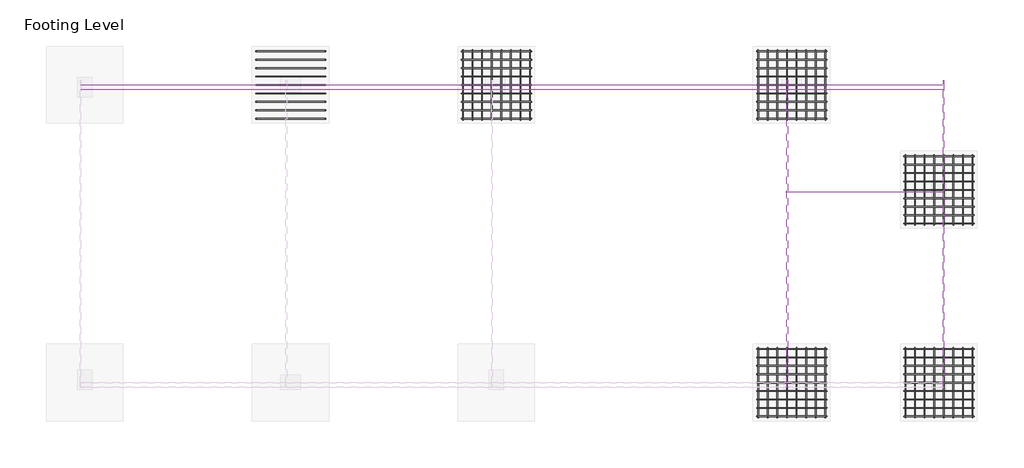
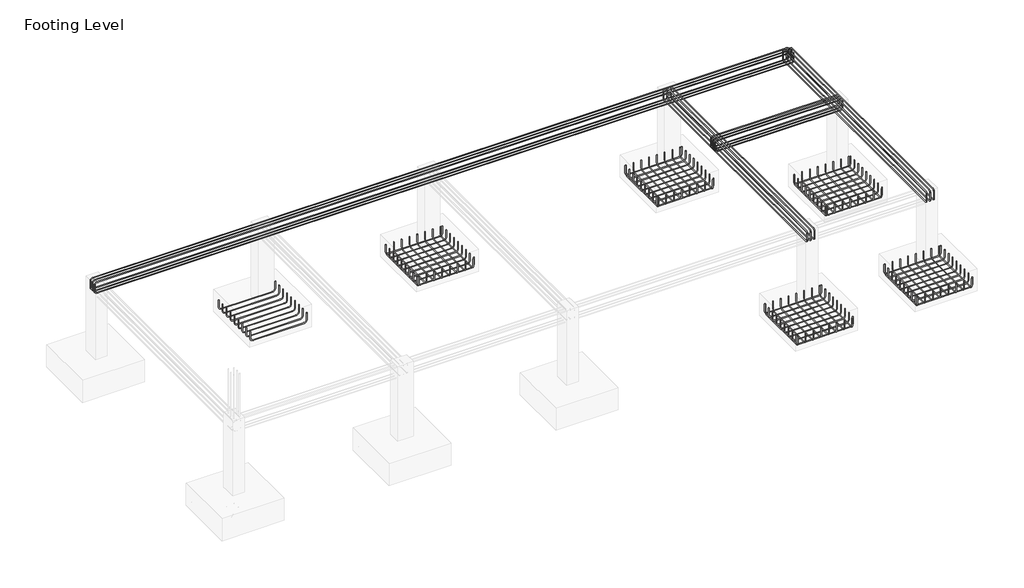
# One storey, part 3 of 3: 19 reinforcing bars.
"""IFC4 building model written with IfcOpenShell, lengths in millimetres."""

from ifc_helpers import new_model, si_unit, point, frame, origin, place, context, project, spatial, polyline, circle_curve, trimmed, segment, composite_curve, source, transform, mapped, element, save
from ifc_brep_helpers import swept_disk

model = new_model("IFC4")

# Units and contexts
model_context = context("Model", 3, world=origin())
ifc_project = project(units=[si_unit("LENGTHUNIT", "METRE", prefix="MILLI")], contexts=[model_context])

# Site, building, storey
site = spatial("IfcSite", under=ifc_project)
building = spatial("IfcBuilding", under=site)
storey = spatial("IfcBuildingStorey", under=building, Name="Footing Level", Elevation=-1524.0)

# Reinforcing bars
placement = place(None, origin())
reinforcing_bar_shape = source(origin(), model_context, "Body", "SolidModel", [
    swept_disk(composite_curve([segment(polyline([(2294.7534193, -243.2665369, -1724.0), (2294.7534193, -243.2665369, -1872.0)]), True, "CONTINUOUS"), segment(trimmed(circle_curve(frame((2294.7534193, -197.2665369, -1872.0), z_axis=(1.0, 0.0, 0.0), x_axis=(0.0, -46.0, 0.0)), 46.0), [point((2294.7534193, -243.2665369, -1872.0))], [point((2294.7534193, -197.2665369, -1918.0))], True, "CARTESIAN"), True, "CONTINUOUS"), segment(polyline([(2294.7534193, -197.2665369, -1918.0), (2294.7534193, 798.7334631, -1918.0)]), True, "CONTINUOUS"), segment(trimmed(circle_curve(frame((2294.7534193, 798.7334631, -1872.0), z_axis=(1.0, 0.0, 0.0), x_axis=(0.0, 0.0, -46.0)), 46.0), [point((2294.7534193, 798.7334631, -1918.0))], [point((2294.7534193, 844.7334631, -1872.0))], True, "CARTESIAN"), True, "CONTINUOUS"), segment(polyline([(2294.7534193, 844.7334631, -1872.0), (2294.7534193, 844.7334631, -1724.0)]), True, "CONTINUOUS")], self_intersect=False), 6.0),
])
element("IfcReinforcingBar", 1, at=placement, inside=storey, context=model_context, shape_type="MappedRepresentation", body=[
    mapped(reinforcing_bar_shape, transform((0.0, 0.0, 0.0), x_axis=(1.0, 0.0, 0.0), y_axis=(0.0, 1.0, 0.0), z_axis=(0.0, 0.0, 1.0))),
    mapped(reinforcing_bar_shape, transform((-149.7374868, 0.0, 0.0), x_axis=(1.0, 0.0, 0.0), y_axis=(0.0, 1.0, 0.0), z_axis=(0.0, 0.0, 1.0))),
    mapped(reinforcing_bar_shape, transform((-299.4749737, 0.0, 0.0), x_axis=(1.0, 0.0, 0.0), y_axis=(0.0, 1.0, 0.0), z_axis=(0.0, 0.0, 1.0))),
    mapped(reinforcing_bar_shape, transform((-449.2124605, 0.0, 0.0), x_axis=(1.0, 0.0, 0.0), y_axis=(0.0, 1.0, 0.0), z_axis=(0.0, 0.0, 1.0))),
    mapped(reinforcing_bar_shape, transform((-598.9499474, 0.0, 0.0), x_axis=(1.0, 0.0, 0.0), y_axis=(0.0, 1.0, 0.0), z_axis=(0.0, 0.0, 1.0))),
    mapped(reinforcing_bar_shape, transform((-748.6874342, 0.0, 0.0), x_axis=(1.0, 0.0, 0.0), y_axis=(0.0, 1.0, 0.0), z_axis=(0.0, 0.0, 1.0))),
    mapped(reinforcing_bar_shape, transform((-898.424921, 0.0, 0.0), x_axis=(1.0, 0.0, 0.0), y_axis=(0.0, 1.0, 0.0), z_axis=(0.0, 0.0, 1.0))),
    mapped(reinforcing_bar_shape, transform((-1048.1624079, 0.0, 0.0), x_axis=(1.0, 0.0, 0.0), y_axis=(0.0, 1.0, 0.0), z_axis=(0.0, 0.0, 1.0))),
])
reinforcing_bar_2_shape = source(origin(), model_context, "Body", "SolidModel", [
    swept_disk(composite_curve([segment(polyline([(1227.6882476, -224.7796689, -1711.15), (1227.6882476, -224.7796689, -1859.15)]), True, "CONTINUOUS"), segment(trimmed(circle_curve(frame((1273.6882476, -224.7796689, -1859.15), z_axis=(0.0, -1.0, 0.0), x_axis=(-46.0, 0.0, 0.0)), 46.0), [point((1227.6882476, -224.7796689, -1859.15))], [point((1273.6882476, -224.7796689, -1905.15))], True, "CARTESIAN"), True, "CONTINUOUS"), segment(polyline([(1273.6882476, -224.7796689, -1905.15), (2269.6882476, -224.7796689, -1905.15)]), True, "CONTINUOUS"), segment(trimmed(circle_curve(frame((2269.6882476, -224.7796689, -1859.15), z_axis=(0.0, -1.0, 0.0), x_axis=(0.0, 0.0, -46.0)), 46.0), [point((2269.6882476, -224.7796689, -1905.15))], [point((2315.6882476, -224.7796689, -1859.15))], True, "CARTESIAN"), True, "CONTINUOUS"), segment(polyline([(2315.6882476, -224.7796689, -1859.15), (2315.6882476, -224.7796689, -1711.15)]), True, "CONTINUOUS")], self_intersect=False), 6.0),
])
element("IfcReinforcingBar", 2, at=placement, inside=storey, context=model_context, shape_type="MappedRepresentation", body=[
    mapped(reinforcing_bar_2_shape, transform((0.0, 0.0, 0.0), x_axis=(1.0, 0.0, 0.0), y_axis=(0.0, 1.0, 0.0), z_axis=(0.0, 0.0, 1.0))),
    mapped(reinforcing_bar_2_shape, transform((0.0, 131.3537501, 0.0), x_axis=(1.0, 0.0, 0.0), y_axis=(0.0, 1.0, 0.0), z_axis=(0.0, 0.0, 1.0))),
    mapped(reinforcing_bar_2_shape, transform((0.0, 262.7075003, 0.0), x_axis=(1.0, 0.0, 0.0), y_axis=(0.0, 1.0, 0.0), z_axis=(0.0, 0.0, 1.0))),
    mapped(reinforcing_bar_2_shape, transform((0.0, 394.0612504, 0.0), x_axis=(1.0, 0.0, 0.0), y_axis=(0.0, 1.0, 0.0), z_axis=(0.0, 0.0, 1.0))),
    mapped(reinforcing_bar_2_shape, transform((0.0, 525.4150006, 0.0), x_axis=(1.0, 0.0, 0.0), y_axis=(0.0, 1.0, 0.0), z_axis=(0.0, 0.0, 1.0))),
    mapped(reinforcing_bar_2_shape, transform((0.0, 656.7687507, 0.0), x_axis=(1.0, 0.0, 0.0), y_axis=(0.0, 1.0, 0.0), z_axis=(0.0, 0.0, 1.0))),
    mapped(reinforcing_bar_2_shape, transform((0.0, 788.1225008, 0.0), x_axis=(1.0, 0.0, 0.0), y_axis=(0.0, 1.0, 0.0), z_axis=(0.0, 0.0, 1.0))),
    mapped(reinforcing_bar_2_shape, transform((0.0, 919.476251, 0.0), x_axis=(1.0, 0.0, 0.0), y_axis=(0.0, 1.0, 0.0), z_axis=(0.0, 0.0, 1.0))),
    mapped(reinforcing_bar_2_shape, transform((0.0, 1050.8300011, 0.0), x_axis=(1.0, 0.0, 0.0), y_axis=(0.0, 1.0, 0.0), z_axis=(0.0, 0.0, 1.0))),
])
reinforcing_bar_3_shape = source(origin(), model_context, "Body", "SolidModel", [
    swept_disk(composite_curve([segment(polyline([(4593.4534193, -243.2665369, -1724.0), (4593.4534193, -243.2665369, -1872.0)]), True, "CONTINUOUS"), segment(trimmed(circle_curve(frame((4593.4534193, -197.2665369, -1872.0), z_axis=(1.0, 0.0, 0.0), x_axis=(0.0, -46.0, 0.0)), 46.0), [point((4593.4534193, -243.2665369, -1872.0))], [point((4593.4534193, -197.2665369, -1918.0))], True, "CARTESIAN"), True, "CONTINUOUS"), segment(polyline([(4593.4534193, -197.2665369, -1918.0), (4593.4534193, 798.7334631, -1918.0)]), True, "CONTINUOUS"), segment(trimmed(circle_curve(frame((4593.4534193, 798.7334631, -1872.0), z_axis=(1.0, 0.0, 0.0), x_axis=(0.0, 0.0, -46.0)), 46.0), [point((4593.4534193, 798.7334631, -1918.0))], [point((4593.4534193, 844.7334631, -1872.0))], True, "CARTESIAN"), True, "CONTINUOUS"), segment(polyline([(4593.4534193, 844.7334631, -1872.0), (4593.4534193, 844.7334631, -1724.0)]), True, "CONTINUOUS")], self_intersect=False), 6.0),
])
element("IfcReinforcingBar", 3, at=placement, inside=storey, context=model_context, shape_type="MappedRepresentation", body=[
    mapped(reinforcing_bar_3_shape, transform((0.0, 0.0, 0.0), x_axis=(1.0, 0.0, 0.0), y_axis=(0.0, 1.0, 0.0), z_axis=(0.0, 0.0, 1.0))),
    mapped(reinforcing_bar_3_shape, transform((-149.7374868, 0.0, 0.0), x_axis=(1.0, 0.0, 0.0), y_axis=(0.0, 1.0, 0.0), z_axis=(0.0, 0.0, 1.0))),
    mapped(reinforcing_bar_3_shape, transform((-299.4749737, 0.0, 0.0), x_axis=(1.0, 0.0, 0.0), y_axis=(0.0, 1.0, 0.0), z_axis=(0.0, 0.0, 1.0))),
    mapped(reinforcing_bar_3_shape, transform((-449.2124605, 0.0, 0.0), x_axis=(1.0, 0.0, 0.0), y_axis=(0.0, 1.0, 0.0), z_axis=(0.0, 0.0, 1.0))),
    mapped(reinforcing_bar_3_shape, transform((-598.9499474, 0.0, 0.0), x_axis=(1.0, 0.0, 0.0), y_axis=(0.0, 1.0, 0.0), z_axis=(0.0, 0.0, 1.0))),
    mapped(reinforcing_bar_3_shape, transform((-748.6874342, 0.0, 0.0), x_axis=(1.0, 0.0, 0.0), y_axis=(0.0, 1.0, 0.0), z_axis=(0.0, 0.0, 1.0))),
    mapped(reinforcing_bar_3_shape, transform((-898.424921, 0.0, 0.0), x_axis=(1.0, 0.0, 0.0), y_axis=(0.0, 1.0, 0.0), z_axis=(0.0, 0.0, 1.0))),
    mapped(reinforcing_bar_3_shape, transform((-1048.1624079, 0.0, 0.0), x_axis=(1.0, 0.0, 0.0), y_axis=(0.0, 1.0, 0.0), z_axis=(0.0, 0.0, 1.0))),
])
reinforcing_bar_4_shape = source(origin(), model_context, "Body", "SolidModel", [
    swept_disk(composite_curve([segment(polyline([(3526.3882476, -224.7796689, -1711.15), (3526.3882476, -224.7796689, -1859.15)]), True, "CONTINUOUS"), segment(trimmed(circle_curve(frame((3572.3882476, -224.7796689, -1859.15), z_axis=(0.0, -1.0, 0.0), x_axis=(-46.0, 0.0, 0.0)), 46.0), [point((3526.3882476, -224.7796689, -1859.15))], [point((3572.3882476, -224.7796689, -1905.15))], True, "CARTESIAN"), True, "CONTINUOUS"), segment(polyline([(3572.3882476, -224.7796689, -1905.15), (4568.3882476, -224.7796689, -1905.15)]), True, "CONTINUOUS"), segment(trimmed(circle_curve(frame((4568.3882476, -224.7796689, -1859.15), z_axis=(0.0, -1.0, 0.0), x_axis=(0.0, 0.0, -46.0)), 46.0), [point((4568.3882476, -224.7796689, -1905.15))], [point((4614.3882476, -224.7796689, -1859.15))], True, "CARTESIAN"), True, "CONTINUOUS"), segment(polyline([(4614.3882476, -224.7796689, -1859.15), (4614.3882476, -224.7796689, -1711.15)]), True, "CONTINUOUS")], self_intersect=False), 6.0),
])
element("IfcReinforcingBar", 4, at=placement, inside=storey, context=model_context, shape_type="MappedRepresentation", body=[
    mapped(reinforcing_bar_4_shape, transform((0.0, 0.0, 0.0), x_axis=(1.0, 0.0, 0.0), y_axis=(0.0, 1.0, 0.0), z_axis=(0.0, 0.0, 1.0))),
    mapped(reinforcing_bar_4_shape, transform((0.0, 131.3537501, 0.0), x_axis=(1.0, 0.0, 0.0), y_axis=(0.0, 1.0, 0.0), z_axis=(0.0, 0.0, 1.0))),
    mapped(reinforcing_bar_4_shape, transform((0.0, 262.7075003, 0.0), x_axis=(1.0, 0.0, 0.0), y_axis=(0.0, 1.0, 0.0), z_axis=(0.0, 0.0, 1.0))),
    mapped(reinforcing_bar_4_shape, transform((0.0, 394.0612504, 0.0), x_axis=(1.0, 0.0, 0.0), y_axis=(0.0, 1.0, 0.0), z_axis=(0.0, 0.0, 1.0))),
    mapped(reinforcing_bar_4_shape, transform((0.0, 525.4150006, 0.0), x_axis=(1.0, 0.0, 0.0), y_axis=(0.0, 1.0, 0.0), z_axis=(0.0, 0.0, 1.0))),
    mapped(reinforcing_bar_4_shape, transform((0.0, 656.7687507, 0.0), x_axis=(1.0, 0.0, 0.0), y_axis=(0.0, 1.0, 0.0), z_axis=(0.0, 0.0, 1.0))),
    mapped(reinforcing_bar_4_shape, transform((0.0, 788.1225008, 0.0), x_axis=(1.0, 0.0, 0.0), y_axis=(0.0, 1.0, 0.0), z_axis=(0.0, 0.0, 1.0))),
    mapped(reinforcing_bar_4_shape, transform((0.0, 919.476251, 0.0), x_axis=(1.0, 0.0, 0.0), y_axis=(0.0, 1.0, 0.0), z_axis=(0.0, 0.0, 1.0))),
    mapped(reinforcing_bar_4_shape, transform((0.0, 1050.8300011, 0.0), x_axis=(1.0, 0.0, 0.0), y_axis=(0.0, 1.0, 0.0), z_axis=(0.0, 0.0, 1.0))),
])
reinforcing_bar_5_shape = source(origin(), model_context, "Body", "SolidModel", [
    swept_disk(composite_curve([segment(polyline([(4593.4534193, 2766.6334631, -1724.0), (4593.4534193, 2766.6334631, -1872.0)]), True, "CONTINUOUS"), segment(trimmed(circle_curve(frame((4593.4534193, 2812.6334631, -1872.0), z_axis=(1.0, 0.0, 0.0), x_axis=(0.0, -46.0, 0.0)), 46.0), [point((4593.4534193, 2766.6334631, -1872.0))], [point((4593.4534193, 2812.6334631, -1918.0))], True, "CARTESIAN"), True, "CONTINUOUS"), segment(polyline([(4593.4534193, 2812.6334631, -1918.0), (4593.4534193, 3808.6334631, -1918.0)]), True, "CONTINUOUS"), segment(trimmed(circle_curve(frame((4593.4534193, 3808.6334631, -1872.0), z_axis=(1.0, 0.0, 0.0), x_axis=(0.0, 0.0, -46.0)), 46.0), [point((4593.4534193, 3808.6334631, -1918.0))], [point((4593.4534193, 3854.6334631, -1872.0))], True, "CARTESIAN"), True, "CONTINUOUS"), segment(polyline([(4593.4534193, 3854.6334631, -1872.0), (4593.4534193, 3854.6334631, -1724.0)]), True, "CONTINUOUS")], self_intersect=False), 6.0),
])
element("IfcReinforcingBar", 5, at=placement, inside=storey, context=model_context, shape_type="MappedRepresentation", body=[
    mapped(reinforcing_bar_5_shape, transform((0.0, 0.0, 0.0), x_axis=(1.0, 0.0, 0.0), y_axis=(0.0, 1.0, 0.0), z_axis=(0.0, 0.0, 1.0))),
    mapped(reinforcing_bar_5_shape, transform((-149.7374868, 0.0, 0.0), x_axis=(1.0, 0.0, 0.0), y_axis=(0.0, 1.0, 0.0), z_axis=(0.0, 0.0, 1.0))),
    mapped(reinforcing_bar_5_shape, transform((-299.4749737, 0.0, 0.0), x_axis=(1.0, 0.0, 0.0), y_axis=(0.0, 1.0, 0.0), z_axis=(0.0, 0.0, 1.0))),
    mapped(reinforcing_bar_5_shape, transform((-449.2124605, 0.0, 0.0), x_axis=(1.0, 0.0, 0.0), y_axis=(0.0, 1.0, 0.0), z_axis=(0.0, 0.0, 1.0))),
    mapped(reinforcing_bar_5_shape, transform((-598.9499474, 0.0, 0.0), x_axis=(1.0, 0.0, 0.0), y_axis=(0.0, 1.0, 0.0), z_axis=(0.0, 0.0, 1.0))),
    mapped(reinforcing_bar_5_shape, transform((-748.6874342, 0.0, 0.0), x_axis=(1.0, 0.0, 0.0), y_axis=(0.0, 1.0, 0.0), z_axis=(0.0, 0.0, 1.0))),
    mapped(reinforcing_bar_5_shape, transform((-898.424921, 0.0, 0.0), x_axis=(1.0, 0.0, 0.0), y_axis=(0.0, 1.0, 0.0), z_axis=(0.0, 0.0, 1.0))),
    mapped(reinforcing_bar_5_shape, transform((-1048.1624079, 0.0, 0.0), x_axis=(1.0, 0.0, 0.0), y_axis=(0.0, 1.0, 0.0), z_axis=(0.0, 0.0, 1.0))),
])
reinforcing_bar_6_shape = source(origin(), model_context, "Body", "SolidModel", [
    swept_disk(composite_curve([segment(polyline([(3526.3882476, 2785.1203311, -1711.15), (3526.3882476, 2785.1203311, -1859.15)]), True, "CONTINUOUS"), segment(trimmed(circle_curve(frame((3572.3882476, 2785.1203311, -1859.15), z_axis=(0.0, -1.0, 0.0), x_axis=(-46.0, 0.0, 0.0)), 46.0), [point((3526.3882476, 2785.1203311, -1859.15))], [point((3572.3882476, 2785.1203311, -1905.15))], True, "CARTESIAN"), True, "CONTINUOUS"), segment(polyline([(3572.3882476, 2785.1203311, -1905.15), (4568.3882476, 2785.1203311, -1905.15)]), True, "CONTINUOUS"), segment(trimmed(circle_curve(frame((4568.3882476, 2785.1203311, -1859.15), z_axis=(0.0, -1.0, 0.0), x_axis=(0.0, 0.0, -46.0)), 46.0), [point((4568.3882476, 2785.1203311, -1905.15))], [point((4614.3882476, 2785.1203311, -1859.15))], True, "CARTESIAN"), True, "CONTINUOUS"), segment(polyline([(4614.3882476, 2785.1203311, -1859.15), (4614.3882476, 2785.1203311, -1711.15)]), True, "CONTINUOUS")], self_intersect=False), 6.0),
])
element("IfcReinforcingBar", 6, at=placement, inside=storey, context=model_context, shape_type="MappedRepresentation", body=[
    mapped(reinforcing_bar_6_shape, transform((0.0, 0.0, 0.0), x_axis=(1.0, 0.0, 0.0), y_axis=(0.0, 1.0, 0.0), z_axis=(0.0, 0.0, 1.0))),
    mapped(reinforcing_bar_6_shape, transform((0.0, 131.3537501, 0.0), x_axis=(1.0, 0.0, 0.0), y_axis=(0.0, 1.0, 0.0), z_axis=(0.0, 0.0, 1.0))),
    mapped(reinforcing_bar_6_shape, transform((0.0, 262.7075003, 0.0), x_axis=(1.0, 0.0, 0.0), y_axis=(0.0, 1.0, 0.0), z_axis=(0.0, 0.0, 1.0))),
    mapped(reinforcing_bar_6_shape, transform((0.0, 394.0612504, 0.0), x_axis=(1.0, 0.0, 0.0), y_axis=(0.0, 1.0, 0.0), z_axis=(0.0, 0.0, 1.0))),
    mapped(reinforcing_bar_6_shape, transform((0.0, 525.4150006, 0.0), x_axis=(1.0, 0.0, 0.0), y_axis=(0.0, 1.0, 0.0), z_axis=(0.0, 0.0, 1.0))),
    mapped(reinforcing_bar_6_shape, transform((0.0, 656.7687507, 0.0), x_axis=(1.0, 0.0, 0.0), y_axis=(0.0, 1.0, 0.0), z_axis=(0.0, 0.0, 1.0))),
    mapped(reinforcing_bar_6_shape, transform((0.0, 788.1225008, 0.0), x_axis=(1.0, 0.0, 0.0), y_axis=(0.0, 1.0, 0.0), z_axis=(0.0, 0.0, 1.0))),
    mapped(reinforcing_bar_6_shape, transform((0.0, 919.476251, 0.0), x_axis=(1.0, 0.0, 0.0), y_axis=(0.0, 1.0, 0.0), z_axis=(0.0, 0.0, 1.0))),
    mapped(reinforcing_bar_6_shape, transform((0.0, 1050.8300011, 0.0), x_axis=(1.0, 0.0, 0.0), y_axis=(0.0, 1.0, 0.0), z_axis=(0.0, 0.0, 1.0))),
])
reinforcing_bar_7_shape = source(origin(), model_context, "Body", "SolidModel", [
    swept_disk(composite_curve([segment(polyline([(2294.7534193, 4404.9334631, -1724.0), (2294.7534193, 4404.9334631, -1872.0)]), True, "CONTINUOUS"), segment(trimmed(circle_curve(frame((2294.7534193, 4450.9334631, -1872.0), z_axis=(1.0, 0.0, 0.0), x_axis=(0.0, -46.0, 0.0)), 46.0), [point((2294.7534193, 4404.9334631, -1872.0))], [point((2294.7534193, 4450.9334631, -1918.0))], True, "CARTESIAN"), True, "CONTINUOUS"), segment(polyline([(2294.7534193, 4450.9334631, -1918.0), (2294.7534193, 5446.9334631, -1918.0)]), True, "CONTINUOUS"), segment(trimmed(circle_curve(frame((2294.7534193, 5446.9334631, -1872.0), z_axis=(1.0, 0.0, 0.0), x_axis=(0.0, 0.0, -46.0)), 46.0), [point((2294.7534193, 5446.9334631, -1918.0))], [point((2294.7534193, 5492.9334631, -1872.0))], True, "CARTESIAN"), True, "CONTINUOUS"), segment(polyline([(2294.7534193, 5492.9334631, -1872.0), (2294.7534193, 5492.9334631, -1724.0)]), True, "CONTINUOUS")], self_intersect=False), 6.0),
])
element("IfcReinforcingBar", 7, at=placement, inside=storey, context=model_context, shape_type="MappedRepresentation", body=[
    mapped(reinforcing_bar_7_shape, transform((0.0, 0.0, 0.0), x_axis=(1.0, 0.0, 0.0), y_axis=(0.0, 1.0, 0.0), z_axis=(0.0, 0.0, 1.0))),
    mapped(reinforcing_bar_7_shape, transform((-149.7374868, 0.0, 0.0), x_axis=(1.0, 0.0, 0.0), y_axis=(0.0, 1.0, 0.0), z_axis=(0.0, 0.0, 1.0))),
    mapped(reinforcing_bar_7_shape, transform((-299.4749737, 0.0, 0.0), x_axis=(1.0, 0.0, 0.0), y_axis=(0.0, 1.0, 0.0), z_axis=(0.0, 0.0, 1.0))),
    mapped(reinforcing_bar_7_shape, transform((-449.2124605, 0.0, 0.0), x_axis=(1.0, 0.0, 0.0), y_axis=(0.0, 1.0, 0.0), z_axis=(0.0, 0.0, 1.0))),
    mapped(reinforcing_bar_7_shape, transform((-598.9499474, 0.0, 0.0), x_axis=(1.0, 0.0, 0.0), y_axis=(0.0, 1.0, 0.0), z_axis=(0.0, 0.0, 1.0))),
    mapped(reinforcing_bar_7_shape, transform((-748.6874342, 0.0, 0.0), x_axis=(1.0, 0.0, 0.0), y_axis=(0.0, 1.0, 0.0), z_axis=(0.0, 0.0, 1.0))),
    mapped(reinforcing_bar_7_shape, transform((-898.424921, 0.0, 0.0), x_axis=(1.0, 0.0, 0.0), y_axis=(0.0, 1.0, 0.0), z_axis=(0.0, 0.0, 1.0))),
    mapped(reinforcing_bar_7_shape, transform((-1048.1624079, 0.0, 0.0), x_axis=(1.0, 0.0, 0.0), y_axis=(0.0, 1.0, 0.0), z_axis=(0.0, 0.0, 1.0))),
])
reinforcing_bar_8_shape = source(origin(), model_context, "Body", "SolidModel", [
    swept_disk(composite_curve([segment(polyline([(1227.6882476, 4423.4203311, -1711.15), (1227.6882476, 4423.4203311, -1859.15)]), True, "CONTINUOUS"), segment(trimmed(circle_curve(frame((1273.6882476, 4423.4203311, -1859.15), z_axis=(0.0, -1.0, 0.0), x_axis=(-46.0, 0.0, 0.0)), 46.0), [point((1227.6882476, 4423.4203311, -1859.15))], [point((1273.6882476, 4423.4203311, -1905.15))], True, "CARTESIAN"), True, "CONTINUOUS"), segment(polyline([(1273.6882476, 4423.4203311, -1905.15), (2269.6882476, 4423.4203311, -1905.15)]), True, "CONTINUOUS"), segment(trimmed(circle_curve(frame((2269.6882476, 4423.4203311, -1859.15), z_axis=(0.0, -1.0, 0.0), x_axis=(0.0, 0.0, -46.0)), 46.0), [point((2269.6882476, 4423.4203311, -1905.15))], [point((2315.6882476, 4423.4203311, -1859.15))], True, "CARTESIAN"), True, "CONTINUOUS"), segment(polyline([(2315.6882476, 4423.4203311, -1859.15), (2315.6882476, 4423.4203311, -1711.15)]), True, "CONTINUOUS")], self_intersect=False), 6.0),
])
element("IfcReinforcingBar", 8, at=placement, inside=storey, context=model_context, shape_type="MappedRepresentation", body=[
    mapped(reinforcing_bar_8_shape, transform((0.0, 0.0, 0.0), x_axis=(1.0, 0.0, 0.0), y_axis=(0.0, 1.0, 0.0), z_axis=(0.0, 0.0, 1.0))),
    mapped(reinforcing_bar_8_shape, transform((0.0, 131.3537501, 0.0), x_axis=(1.0, 0.0, 0.0), y_axis=(0.0, 1.0, 0.0), z_axis=(0.0, 0.0, 1.0))),
    mapped(reinforcing_bar_8_shape, transform((0.0, 262.7075003, 0.0), x_axis=(1.0, 0.0, 0.0), y_axis=(0.0, 1.0, 0.0), z_axis=(0.0, 0.0, 1.0))),
    mapped(reinforcing_bar_8_shape, transform((0.0, 394.0612504, 0.0), x_axis=(1.0, 0.0, 0.0), y_axis=(0.0, 1.0, 0.0), z_axis=(0.0, 0.0, 1.0))),
    mapped(reinforcing_bar_8_shape, transform((0.0, 525.4150006, 0.0), x_axis=(1.0, 0.0, 0.0), y_axis=(0.0, 1.0, 0.0), z_axis=(0.0, 0.0, 1.0))),
    mapped(reinforcing_bar_8_shape, transform((0.0, 656.7687507, 0.0), x_axis=(1.0, 0.0, 0.0), y_axis=(0.0, 1.0, 0.0), z_axis=(0.0, 0.0, 1.0))),
    mapped(reinforcing_bar_8_shape, transform((0.0, 788.1225008, 0.0), x_axis=(1.0, 0.0, 0.0), y_axis=(0.0, 1.0, 0.0), z_axis=(0.0, 0.0, 1.0))),
    mapped(reinforcing_bar_8_shape, transform((0.0, 919.476251, 0.0), x_axis=(1.0, 0.0, 0.0), y_axis=(0.0, 1.0, 0.0), z_axis=(0.0, 0.0, 1.0))),
    mapped(reinforcing_bar_8_shape, transform((0.0, 1050.8300011, 0.0), x_axis=(1.0, 0.0, 0.0), y_axis=(0.0, 1.0, 0.0), z_axis=(0.0, 0.0, 1.0))),
])
reinforcing_bar_9_shape = source(origin(), model_context, "Body", "SolidModel", [
    swept_disk(composite_curve([segment(polyline([(-2315.3465807, 4404.9334631, -1724.0), (-2315.3465807, 4404.9334631, -1872.0)]), True, "CONTINUOUS"), segment(trimmed(circle_curve(frame((-2315.3465807, 4450.9334631, -1872.0), z_axis=(1.0, 0.0, 0.0), x_axis=(0.0, -46.0, 0.0)), 46.0), [point((-2315.3465807, 4404.9334631, -1872.0))], [point((-2315.3465807, 4450.9334631, -1918.0))], True, "CARTESIAN"), True, "CONTINUOUS"), segment(polyline([(-2315.3465807, 4450.9334631, -1918.0), (-2315.3465807, 5446.9334631, -1918.0)]), True, "CONTINUOUS"), segment(trimmed(circle_curve(frame((-2315.3465807, 5446.9334631, -1872.0), z_axis=(1.0, 0.0, 0.0), x_axis=(0.0, 0.0, -46.0)), 46.0), [point((-2315.3465807, 5446.9334631, -1918.0))], [point((-2315.3465807, 5492.9334631, -1872.0))], True, "CARTESIAN"), True, "CONTINUOUS"), segment(polyline([(-2315.3465807, 5492.9334631, -1872.0), (-2315.3465807, 5492.9334631, -1724.0)]), True, "CONTINUOUS")], self_intersect=False), 6.0),
])
element("IfcReinforcingBar", 9, at=placement, inside=storey, context=model_context, shape_type="MappedRepresentation", body=[
    mapped(reinforcing_bar_9_shape, transform((0.0, 0.0, 0.0), x_axis=(1.0, 0.0, 0.0), y_axis=(0.0, 1.0, 0.0), z_axis=(0.0, 0.0, 1.0))),
    mapped(reinforcing_bar_9_shape, transform((-149.7374868, 0.0, 0.0), x_axis=(1.0, 0.0, 0.0), y_axis=(0.0, 1.0, 0.0), z_axis=(0.0, 0.0, 1.0))),
    mapped(reinforcing_bar_9_shape, transform((-299.4749737, 0.0, 0.0), x_axis=(1.0, 0.0, 0.0), y_axis=(0.0, 1.0, 0.0), z_axis=(0.0, 0.0, 1.0))),
    mapped(reinforcing_bar_9_shape, transform((-449.2124605, 0.0, 0.0), x_axis=(1.0, 0.0, 0.0), y_axis=(0.0, 1.0, 0.0), z_axis=(0.0, 0.0, 1.0))),
    mapped(reinforcing_bar_9_shape, transform((-598.9499474, 0.0, 0.0), x_axis=(1.0, 0.0, 0.0), y_axis=(0.0, 1.0, 0.0), z_axis=(0.0, 0.0, 1.0))),
    mapped(reinforcing_bar_9_shape, transform((-748.6874342, 0.0, 0.0), x_axis=(1.0, 0.0, 0.0), y_axis=(0.0, 1.0, 0.0), z_axis=(0.0, 0.0, 1.0))),
    mapped(reinforcing_bar_9_shape, transform((-898.424921, 0.0, 0.0), x_axis=(1.0, 0.0, 0.0), y_axis=(0.0, 1.0, 0.0), z_axis=(0.0, 0.0, 1.0))),
    mapped(reinforcing_bar_9_shape, transform((-1048.1624079, 0.0, 0.0), x_axis=(1.0, 0.0, 0.0), y_axis=(0.0, 1.0, 0.0), z_axis=(0.0, 0.0, 1.0))),
])
reinforcing_bar_10_shape = source(origin(), model_context, "Body", "SolidModel", [
    swept_disk(composite_curve([segment(polyline([(-3382.4117524, 4423.4203311, -1711.15), (-3382.4117524, 4423.4203311, -1859.15)]), True, "CONTINUOUS"), segment(trimmed(circle_curve(frame((-3336.4117524, 4423.4203311, -1859.15), z_axis=(0.0, -1.0, 0.0), x_axis=(-46.0, 0.0, 0.0)), 46.0), [point((-3382.4117524, 4423.4203311, -1859.15))], [point((-3336.4117524, 4423.4203311, -1905.15))], True, "CARTESIAN"), True, "CONTINUOUS"), segment(polyline([(-3336.4117524, 4423.4203311, -1905.15), (-2340.4117524, 4423.4203311, -1905.15)]), True, "CONTINUOUS"), segment(trimmed(circle_curve(frame((-2340.4117524, 4423.4203311, -1859.15), z_axis=(0.0, -1.0, 0.0), x_axis=(0.0, 0.0, -46.0)), 46.0), [point((-2340.4117524, 4423.4203311, -1905.15))], [point((-2294.4117524, 4423.4203311, -1859.15))], True, "CARTESIAN"), True, "CONTINUOUS"), segment(polyline([(-2294.4117524, 4423.4203311, -1859.15), (-2294.4117524, 4423.4203311, -1711.15)]), True, "CONTINUOUS")], self_intersect=False), 6.0),
])
element("IfcReinforcingBar", 10, at=placement, inside=storey, context=model_context, shape_type="MappedRepresentation", body=[
    mapped(reinforcing_bar_10_shape, transform((0.0, 0.0, 0.0), x_axis=(1.0, 0.0, 0.0), y_axis=(0.0, 1.0, 0.0), z_axis=(0.0, 0.0, 1.0))),
    mapped(reinforcing_bar_10_shape, transform((0.0, 131.3537501, 0.0), x_axis=(1.0, 0.0, 0.0), y_axis=(0.0, 1.0, 0.0), z_axis=(0.0, 0.0, 1.0))),
    mapped(reinforcing_bar_10_shape, transform((0.0, 262.7075003, 0.0), x_axis=(1.0, 0.0, 0.0), y_axis=(0.0, 1.0, 0.0), z_axis=(0.0, 0.0, 1.0))),
    mapped(reinforcing_bar_10_shape, transform((0.0, 394.0612504, 0.0), x_axis=(1.0, 0.0, 0.0), y_axis=(0.0, 1.0, 0.0), z_axis=(0.0, 0.0, 1.0))),
    mapped(reinforcing_bar_10_shape, transform((0.0, 525.4150006, 0.0), x_axis=(1.0, 0.0, 0.0), y_axis=(0.0, 1.0, 0.0), z_axis=(0.0, 0.0, 1.0))),
    mapped(reinforcing_bar_10_shape, transform((0.0, 656.7687507, 0.0), x_axis=(1.0, 0.0, 0.0), y_axis=(0.0, 1.0, 0.0), z_axis=(0.0, 0.0, 1.0))),
    mapped(reinforcing_bar_10_shape, transform((0.0, 788.1225008, 0.0), x_axis=(1.0, 0.0, 0.0), y_axis=(0.0, 1.0, 0.0), z_axis=(0.0, 0.0, 1.0))),
    mapped(reinforcing_bar_10_shape, transform((0.0, 919.476251, 0.0), x_axis=(1.0, 0.0, 0.0), y_axis=(0.0, 1.0, 0.0), z_axis=(0.0, 0.0, 1.0))),
    mapped(reinforcing_bar_10_shape, transform((0.0, 1050.8300011, 0.0), x_axis=(1.0, 0.0, 0.0), y_axis=(0.0, 1.0, 0.0), z_axis=(0.0, 0.0, 1.0))),
])
reinforcing_bar_11_shape = source(origin(), model_context, "Body", "SolidModel", [
    swept_disk(composite_curve([segment(polyline([(-6595.5117524, 4423.4203311, -1711.15), (-6595.5117524, 4423.4203311, -1859.15)]), True, "CONTINUOUS"), segment(trimmed(circle_curve(frame((-6549.5117524, 4423.4203311, -1859.15), z_axis=(0.0, -1.0, 0.0), x_axis=(-46.0, 0.0, 0.0)), 46.0), [point((-6595.5117524, 4423.4203311, -1859.15))], [point((-6549.5117524, 4423.4203311, -1905.15))], True, "CARTESIAN"), True, "CONTINUOUS"), segment(polyline([(-6549.5117524, 4423.4203311, -1905.15), (-5553.5117524, 4423.4203311, -1905.15)]), True, "CONTINUOUS"), segment(trimmed(circle_curve(frame((-5553.5117524, 4423.4203311, -1859.15), z_axis=(0.0, -1.0, 0.0), x_axis=(0.0, 0.0, -46.0)), 46.0), [point((-5553.5117524, 4423.4203311, -1905.15))], [point((-5507.5117524, 4423.4203311, -1859.15))], True, "CARTESIAN"), True, "CONTINUOUS"), segment(polyline([(-5507.5117524, 4423.4203311, -1859.15), (-5507.5117524, 4423.4203311, -1711.15)]), True, "CONTINUOUS")], self_intersect=False), 6.0),
])
element("IfcReinforcingBar", 11, at=placement, inside=storey, context=model_context, shape_type="MappedRepresentation", body=[
    mapped(reinforcing_bar_11_shape, transform((0.0, 0.0, 0.0), x_axis=(1.0, 0.0, 0.0), y_axis=(0.0, 1.0, 0.0), z_axis=(0.0, 0.0, 1.0))),
    mapped(reinforcing_bar_11_shape, transform((0.0, 131.3537501, 0.0), x_axis=(1.0, 0.0, 0.0), y_axis=(0.0, 1.0, 0.0), z_axis=(0.0, 0.0, 1.0))),
    mapped(reinforcing_bar_11_shape, transform((0.0, 262.7075003, 0.0), x_axis=(1.0, 0.0, 0.0), y_axis=(0.0, 1.0, 0.0), z_axis=(0.0, 0.0, 1.0))),
    mapped(reinforcing_bar_11_shape, transform((0.0, 394.0612504, 0.0), x_axis=(1.0, 0.0, 0.0), y_axis=(0.0, 1.0, 0.0), z_axis=(0.0, 0.0, 1.0))),
    mapped(reinforcing_bar_11_shape, transform((0.0, 525.4150006, 0.0), x_axis=(1.0, 0.0, 0.0), y_axis=(0.0, 1.0, 0.0), z_axis=(0.0, 0.0, 1.0))),
    mapped(reinforcing_bar_11_shape, transform((0.0, 656.7687507, 0.0), x_axis=(1.0, 0.0, 0.0), y_axis=(0.0, 1.0, 0.0), z_axis=(0.0, 0.0, 1.0))),
    mapped(reinforcing_bar_11_shape, transform((0.0, 788.1225008, 0.0), x_axis=(1.0, 0.0, 0.0), y_axis=(0.0, 1.0, 0.0), z_axis=(0.0, 0.0, 1.0))),
    mapped(reinforcing_bar_11_shape, transform((0.0, 919.476251, 0.0), x_axis=(1.0, 0.0, 0.0), y_axis=(0.0, 1.0, 0.0), z_axis=(0.0, 0.0, 1.0))),
    mapped(reinforcing_bar_11_shape, transform((0.0, 1050.8300011, 0.0), x_axis=(1.0, 0.0, 0.0), y_axis=(0.0, 1.0, 0.0), z_axis=(0.0, 0.0, 1.0))),
])
reinforcing_bar_12_shape = source(origin(), model_context, "Body", "SolidModel", [
    swept_disk(composite_curve([segment(polyline([(1700.4887526, 5017.2334631, -237.1005051), (1700.4887526, 5017.2334631, -89.1005051)]), True, "CONTINUOUS"), segment(trimmed(circle_curve(frame((1700.4887526, 4971.2334631, -89.1005051), z_axis=(1.0, 0.0, 0.0), x_axis=(0.0, 46.0, 0.0)), 46.0), [point((1700.4887526, 5017.2334631, -89.1005051))], [point((1700.4887526, 4971.2334631, -43.1005051))], True, "CARTESIAN"), True, "CONTINUOUS"), segment(polyline([(1700.4887526, 4971.2334631, -43.1005051), (1700.4887526, 278.4334631, -43.1005051)]), True, "CONTINUOUS"), segment(trimmed(circle_curve(frame((1700.4887526, 278.4334631, -89.1005051), z_axis=(1.0, 0.0, 0.0), x_axis=(0.0, 0.0, 46.00000000000001)), 46.0), [point((1700.4887526, 278.4334631, -43.1005051))], [point((1700.4887526, 232.4334631, -89.1005051))], True, "CARTESIAN"), True, "CONTINUOUS"), segment(polyline([(1700.4887526, 232.4334631, -89.1005051), (1700.4887526, 232.4334631, -237.1005051)]), True, "CONTINUOUS")], self_intersect=False), 6.0),
])
element("IfcReinforcingBar", 12, at=placement, inside=storey, context=model_context, shape_type="MappedRepresentation", body=[
    mapped(reinforcing_bar_12_shape, transform((0.0, 0.0, 0.0), x_axis=(1.0, 0.0, 0.0), y_axis=(0.0, 1.0, 0.0), z_axis=(0.0, 0.0, 1.0))),
    mapped(reinforcing_bar_12_shape, transform((71.1994949, 0.0, 0.0), x_axis=(1.0, 0.0, 0.0), y_axis=(0.0, 1.0, 0.0), z_axis=(0.0, 0.0, 1.0))),
    mapped(reinforcing_bar_12_shape, transform((142.3989899, 0.0, 0.0), x_axis=(1.0, 0.0, 0.0), y_axis=(0.0, 1.0, 0.0), z_axis=(0.0, 0.0, 1.0))),
])
reinforcing_bar_13_shape = source(origin(), model_context, "Body", "SolidModel", [
    swept_disk(composite_curve([segment(polyline([(1700.4887526, 5017.2334631, -67.6994949), (1700.4887526, 5017.2334631, -215.6994949)]), True, "CONTINUOUS"), segment(trimmed(circle_curve(frame((1700.4887526, 4971.2334631, -215.6994949), z_axis=(-1.0, 0.0, 0.0), x_axis=(0.0, 46.0, 0.0)), 46.0), [point((1700.4887526, 5017.2334631, -215.6994949))], [point((1700.4887526, 4971.2334631, -261.6994949))], True, "CARTESIAN"), True, "CONTINUOUS"), segment(polyline([(1700.4887526, 4971.2334631, -261.6994949), (1700.4887526, 278.4334631, -261.6994949)]), True, "CONTINUOUS"), segment(trimmed(circle_curve(frame((1700.4887526, 278.4334631, -215.6994949), z_axis=(-1.0, 0.0, 0.0), x_axis=(0.0, 0.0, -46.0)), 46.0), [point((1700.4887526, 278.4334631, -261.6994949))], [point((1700.4887526, 232.4334631, -215.6994949))], True, "CARTESIAN"), True, "CONTINUOUS"), segment(polyline([(1700.4887526, 232.4334631, -215.6994949), (1700.4887526, 232.4334631, -67.6994949)]), True, "CONTINUOUS")], self_intersect=False), 6.0),
])
element("IfcReinforcingBar", 13, at=placement, inside=storey, context=model_context, shape_type="MappedRepresentation", body=[
    mapped(reinforcing_bar_13_shape, transform((0.0, 0.0, 0.0), x_axis=(1.0, 0.0, 0.0), y_axis=(0.0, 1.0, 0.0), z_axis=(0.0, 0.0, 1.0))),
    mapped(reinforcing_bar_13_shape, transform((71.1994949, 0.0, 0.0), x_axis=(1.0, 0.0, 0.0), y_axis=(0.0, 1.0, 0.0), z_axis=(0.0, 0.0, 1.0))),
    mapped(reinforcing_bar_13_shape, transform((142.3989899, 0.0, 0.0), x_axis=(1.0, 0.0, 0.0), y_axis=(0.0, 1.0, 0.0), z_axis=(0.0, 0.0, 1.0))),
])
reinforcing_bar_14_shape = source(origin(), model_context, "Body", "SolidModel", [
    swept_disk(composite_curve([segment(polyline([(3999.1887526, 5017.2334631, -237.1005051), (3999.1887526, 5017.2334631, -89.1005051)]), True, "CONTINUOUS"), segment(trimmed(circle_curve(frame((3999.1887526, 4971.2334631, -89.1005051), z_axis=(1.0, 0.0, 0.0), x_axis=(0.0, 46.0, 0.0)), 46.0), [point((3999.1887526, 5017.2334631, -89.1005051))], [point((3999.1887526, 4971.2334631, -43.1005051))], True, "CARTESIAN"), True, "CONTINUOUS"), segment(polyline([(3999.1887526, 4971.2334631, -43.1005051), (3999.1887526, 278.4334631, -43.1005051)]), True, "CONTINUOUS"), segment(trimmed(circle_curve(frame((3999.1887526, 278.4334631, -89.1005051), z_axis=(1.0, 0.0, 0.0), x_axis=(0.0, 0.0, 46.00000000000001)), 46.0), [point((3999.1887526, 278.4334631, -43.1005051))], [point((3999.1887526, 232.4334631, -89.1005051))], True, "CARTESIAN"), True, "CONTINUOUS"), segment(polyline([(3999.1887526, 232.4334631, -89.1005051), (3999.1887526, 232.4334631, -237.1005051)]), True, "CONTINUOUS")], self_intersect=False), 6.0),
])
element("IfcReinforcingBar", 14, at=placement, inside=storey, context=model_context, shape_type="MappedRepresentation", body=[
    mapped(reinforcing_bar_14_shape, transform((0.0, 0.0, 0.0), x_axis=(1.0, 0.0, 0.0), y_axis=(0.0, 1.0, 0.0), z_axis=(0.0, 0.0, 1.0))),
    mapped(reinforcing_bar_14_shape, transform((71.1994949, 0.0, 0.0), x_axis=(1.0, 0.0, 0.0), y_axis=(0.0, 1.0, 0.0), z_axis=(0.0, 0.0, 1.0))),
    mapped(reinforcing_bar_14_shape, transform((142.3989899, 0.0, 0.0), x_axis=(1.0, 0.0, 0.0), y_axis=(0.0, 1.0, 0.0), z_axis=(0.0, 0.0, 1.0))),
])
reinforcing_bar_15_shape = source(origin(), model_context, "Body", "SolidModel", [
    swept_disk(composite_curve([segment(polyline([(3999.1887526, 5017.2334631, -67.6994949), (3999.1887526, 5017.2334631, -215.6994949)]), True, "CONTINUOUS"), segment(trimmed(circle_curve(frame((3999.1887526, 4971.2334631, -215.6994949), z_axis=(-1.0, 0.0, 0.0), x_axis=(0.0, 46.0, 0.0)), 46.0), [point((3999.1887526, 5017.2334631, -215.6994949))], [point((3999.1887526, 4971.2334631, -261.6994949))], True, "CARTESIAN"), True, "CONTINUOUS"), segment(polyline([(3999.1887526, 4971.2334631, -261.6994949), (3999.1887526, 278.4334631, -261.6994949)]), True, "CONTINUOUS"), segment(trimmed(circle_curve(frame((3999.1887526, 278.4334631, -215.6994949), z_axis=(-1.0, 0.0, 0.0), x_axis=(0.0, 0.0, -46.0)), 46.0), [point((3999.1887526, 278.4334631, -261.6994949))], [point((3999.1887526, 232.4334631, -215.6994949))], True, "CARTESIAN"), True, "CONTINUOUS"), segment(polyline([(3999.1887526, 232.4334631, -215.6994949), (3999.1887526, 232.4334631, -67.6994949)]), True, "CONTINUOUS")], self_intersect=False), 6.0),
])
element("IfcReinforcingBar", 15, at=placement, inside=storey, context=model_context, shape_type="MappedRepresentation", body=[
    mapped(reinforcing_bar_15_shape, transform((0.0, 0.0, 0.0), x_axis=(1.0, 0.0, 0.0), y_axis=(0.0, 1.0, 0.0), z_axis=(0.0, 0.0, 1.0))),
    mapped(reinforcing_bar_15_shape, transform((71.1994949, 0.0, 0.0), x_axis=(1.0, 0.0, 0.0), y_axis=(0.0, 1.0, 0.0), z_axis=(0.0, 0.0, 1.0))),
    mapped(reinforcing_bar_15_shape, transform((142.3989899, 0.0, 0.0), x_axis=(1.0, 0.0, 0.0), y_axis=(0.0, 1.0, 0.0), z_axis=(0.0, 0.0, 1.0))),
])
reinforcing_bar_16_shape = source(origin(), model_context, "Body", "SolidModel", [
    swept_disk(composite_curve([segment(polyline([(-9325.7296265, 4877.7339681, -237.1005051), (-9325.7296265, 4877.7339681, -89.1005051)]), True, "CONTINUOUS"), segment(trimmed(circle_curve(frame((-9279.7296265, 4877.7339681, -89.1005051), z_axis=(0.0, 1.0, 0.0), x_axis=(-46.0, 0.0, 0.0)), 46.0), [point((-9325.7296265, 4877.7339681, -89.1005051))], [point((-9279.7296265, 4877.7339681, -43.1005051))], True, "CARTESIAN"), True, "CONTINUOUS"), segment(polyline([(-9279.7296265, 4877.7339681, -43.1005051), (4070.8650323, 4877.7339681, -43.1005051)]), True, "CONTINUOUS"), segment(trimmed(circle_curve(frame((4070.8650323, 4877.7339681, -89.1005051), z_axis=(0.0, 1.0, 0.0), x_axis=(0.0, 0.0, 46.00000000000001)), 46.0), [point((4070.8650323, 4877.7339681, -43.1005051))], [point((4116.8650323, 4877.7339681, -89.1005051))], True, "CARTESIAN"), True, "CONTINUOUS"), segment(polyline([(4116.8650323, 4877.7339681, -89.1005051), (4116.8650323, 4877.7339681, -237.1005051)]), True, "CONTINUOUS")], self_intersect=False), 6.0),
])
element("IfcReinforcingBar", 16, at=placement, inside=storey, context=model_context, shape_type="MappedRepresentation", body=[
    mapped(reinforcing_bar_16_shape, transform((0.0, 0.0, 0.0), x_axis=(1.0, 0.0, 0.0), y_axis=(0.0, 1.0, 0.0), z_axis=(0.0, 0.0, 1.0))),
    mapped(reinforcing_bar_16_shape, transform((0.0, 71.1994949, 0.0), x_axis=(1.0, 0.0, 0.0), y_axis=(0.0, 1.0, 0.0), z_axis=(0.0, 0.0, 1.0))),
    mapped(reinforcing_bar_16_shape, transform((0.0, 142.3989899, 0.0), x_axis=(1.0, 0.0, 0.0), y_axis=(0.0, 1.0, 0.0), z_axis=(0.0, 0.0, 1.0))),
])
reinforcing_bar_17_shape = source(origin(), model_context, "Body", "SolidModel", [
    swept_disk(composite_curve([segment(polyline([(-9326.1203644, 4877.7339681, -67.6994949), (-9326.1203644, 4877.7339681, -215.6994949)]), True, "CONTINUOUS"), segment(trimmed(circle_curve(frame((-9280.1203644, 4877.7339681, -215.6994949), z_axis=(0.0, -1.0, 0.0), x_axis=(-46.0, 0.0, 0.0)), 46.0), [point((-9326.1203644, 4877.7339681, -215.6994949))], [point((-9280.1203644, 4877.7339681, -261.6994949))], True, "CARTESIAN"), True, "CONTINUOUS"), segment(polyline([(-9280.1203644, 4877.7339681, -261.6994949), (4076.5679264, 4877.7339681, -261.6994949)]), True, "CONTINUOUS"), segment(trimmed(circle_curve(frame((4076.5679264, 4877.7339681, -215.6994949), z_axis=(0.0, -1.0, 0.0), x_axis=(0.0, 0.0, -46.0)), 46.0), [point((4076.5679264, 4877.7339681, -261.6994949))], [point((4122.5679264, 4877.7339681, -215.6994949))], True, "CARTESIAN"), True, "CONTINUOUS"), segment(polyline([(4122.5679264, 4877.7339681, -215.6994949), (4122.5679264, 4877.7339681, -67.6994949)]), True, "CONTINUOUS")], self_intersect=False), 6.0),
])
element("IfcReinforcingBar", 17, at=placement, inside=storey, context=model_context, shape_type="MappedRepresentation", body=[
    mapped(reinforcing_bar_17_shape, transform((0.0, 0.0, 0.0), x_axis=(1.0, 0.0, 0.0), y_axis=(0.0, 1.0, 0.0), z_axis=(0.0, 0.0, 1.0))),
    mapped(reinforcing_bar_17_shape, transform((0.0, 71.1994949, 0.0), x_axis=(1.0, 0.0, 0.0), y_axis=(0.0, 1.0, 0.0), z_axis=(0.0, 0.0, 1.0))),
    mapped(reinforcing_bar_17_shape, transform((0.0, 142.3989899, 0.0), x_axis=(1.0, 0.0, 0.0), y_axis=(0.0, 1.0, 0.0), z_axis=(0.0, 0.0, 1.0))),
])
reinforcing_bar_18_shape = source(origin(), model_context, "Body", "SolidModel", [
    swept_disk(composite_curve([segment(polyline([(4138.6882476, 3279.2814555, -238.8479924), (4138.6882476, 3279.2814555, -90.8479924)]), True, "CONTINUOUS"), segment(trimmed(circle_curve(frame((4092.6882476, 3279.2814555, -90.8479924), z_axis=(0.0, -1.0, 0.0), x_axis=(46.0, 0.0, 0.0)), 46.0), [point((4138.6882476, 3279.2814555, -90.8479924))], [point((4092.6882476, 3279.2814555, -44.8479924))], True, "CARTESIAN"), True, "CONTINUOUS"), segment(polyline([(4092.6882476, 3279.2814555, -44.8479924), (1734.3882476, 3279.2814555, -44.8479924)]), True, "CONTINUOUS"), segment(trimmed(circle_curve(frame((1734.3882476, 3279.2814555, -90.8479924), z_axis=(0.0, -1.0, 0.0), x_axis=(0.0, 0.0, 45.99999999999999)), 46.0), [point((1734.3882476, 3279.2814555, -44.8479924))], [point((1688.3882476, 3279.2814555, -90.8479924))], True, "CARTESIAN"), True, "CONTINUOUS"), segment(polyline([(1688.3882476, 3279.2814555, -90.8479924), (1688.3882476, 3279.2814555, -238.8479924)]), True, "CONTINUOUS")], self_intersect=False), 6.0),
])
element("IfcReinforcingBar", 18, at=placement, inside=storey, context=model_context, shape_type="MappedRepresentation", body=[
    mapped(reinforcing_bar_18_shape, transform((0.0, 0.0, 0.0), x_axis=(1.0, 0.0, 0.0), y_axis=(0.0, 1.0, 0.0), z_axis=(0.0, 0.0, 1.0))),
    mapped(reinforcing_bar_18_shape, transform((0.0, 69.4520076, 0.0), x_axis=(1.0, 0.0, 0.0), y_axis=(0.0, 1.0, 0.0), z_axis=(0.0, 0.0, 1.0))),
    mapped(reinforcing_bar_18_shape, transform((0.0, 138.9040151, 0.0), x_axis=(1.0, 0.0, 0.0), y_axis=(0.0, 1.0, 0.0), z_axis=(0.0, 0.0, 1.0))),
])
reinforcing_bar_19_shape = source(origin(), model_context, "Body", "SolidModel", [
    swept_disk(composite_curve([segment(polyline([(4138.6882476, 3279.2814555, -65.9520076), (4138.6882476, 3279.2814555, -213.9520076)]), True, "CONTINUOUS"), segment(trimmed(circle_curve(frame((4092.6882476, 3279.2814555, -213.9520076), z_axis=(0.0, 1.0, 0.0), x_axis=(46.0, 0.0, 0.0)), 46.0), [point((4138.6882476, 3279.2814555, -213.9520076))], [point((4092.6882476, 3279.2814555, -259.9520076))], True, "CARTESIAN"), True, "CONTINUOUS"), segment(polyline([(4092.6882476, 3279.2814555, -259.9520076), (1734.3882476, 3279.2814555, -259.9520076)]), True, "CONTINUOUS"), segment(trimmed(circle_curve(frame((1734.3882476, 3279.2814555, -213.9520076), z_axis=(0.0, 1.0, 0.0), x_axis=(0.0, 0.0, -46.0)), 46.0), [point((1734.3882476, 3279.2814555, -259.9520076))], [point((1688.3882476, 3279.2814555, -213.9520076))], True, "CARTESIAN"), True, "CONTINUOUS"), segment(polyline([(1688.3882476, 3279.2814555, -213.9520076), (1688.3882476, 3279.2814555, -65.9520076)]), True, "CONTINUOUS")], self_intersect=False), 6.0),
])
element("IfcReinforcingBar", 19, at=placement, inside=storey, context=model_context, shape_type="MappedRepresentation", body=[
    mapped(reinforcing_bar_19_shape, transform((0.0, 0.0, 0.0), x_axis=(1.0, 0.0, 0.0), y_axis=(0.0, 1.0, 0.0), z_axis=(0.0, 0.0, 1.0))),
    mapped(reinforcing_bar_19_shape, transform((0.0, 69.4520076, 0.0), x_axis=(1.0, 0.0, 0.0), y_axis=(0.0, 1.0, 0.0), z_axis=(0.0, 0.0, 1.0))),
    mapped(reinforcing_bar_19_shape, transform((0.0, 138.9040151, 0.0), x_axis=(1.0, 0.0, 0.0), y_axis=(0.0, 1.0, 0.0), z_axis=(0.0, 0.0, 1.0))),
])

save(model, "model.ifc")

# Revit data of these elements
# Elements 1, 2, 3, 4, 5, 6, 7, 8, 9, 10, 11, 12, 13, 14, 15, 16, 17, 18, 19 (IfcReinforcingBar)
#   Phase Created = New Construction
